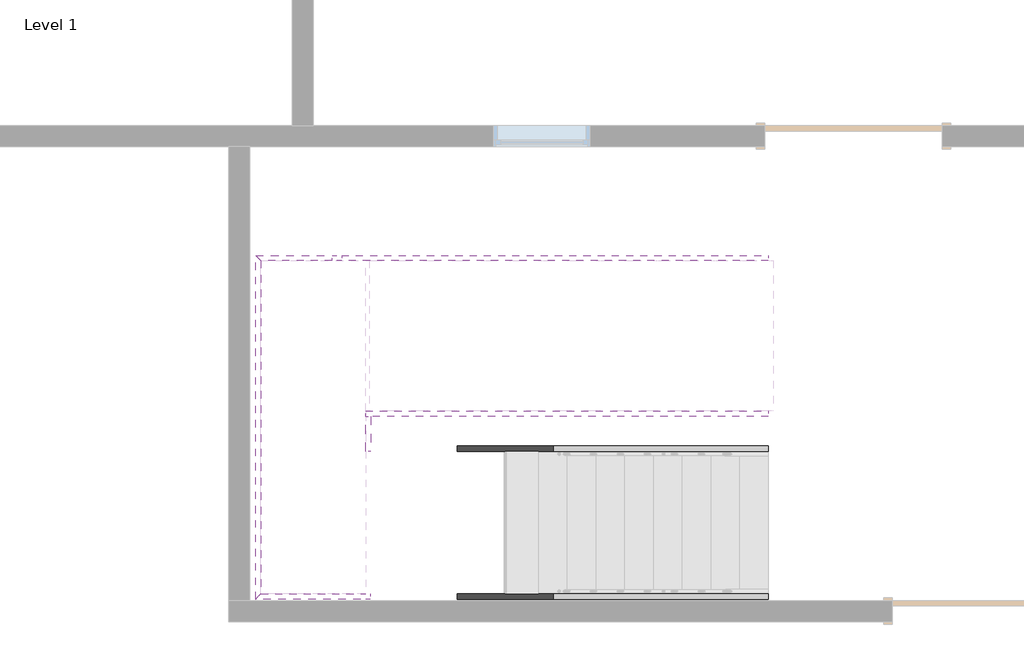
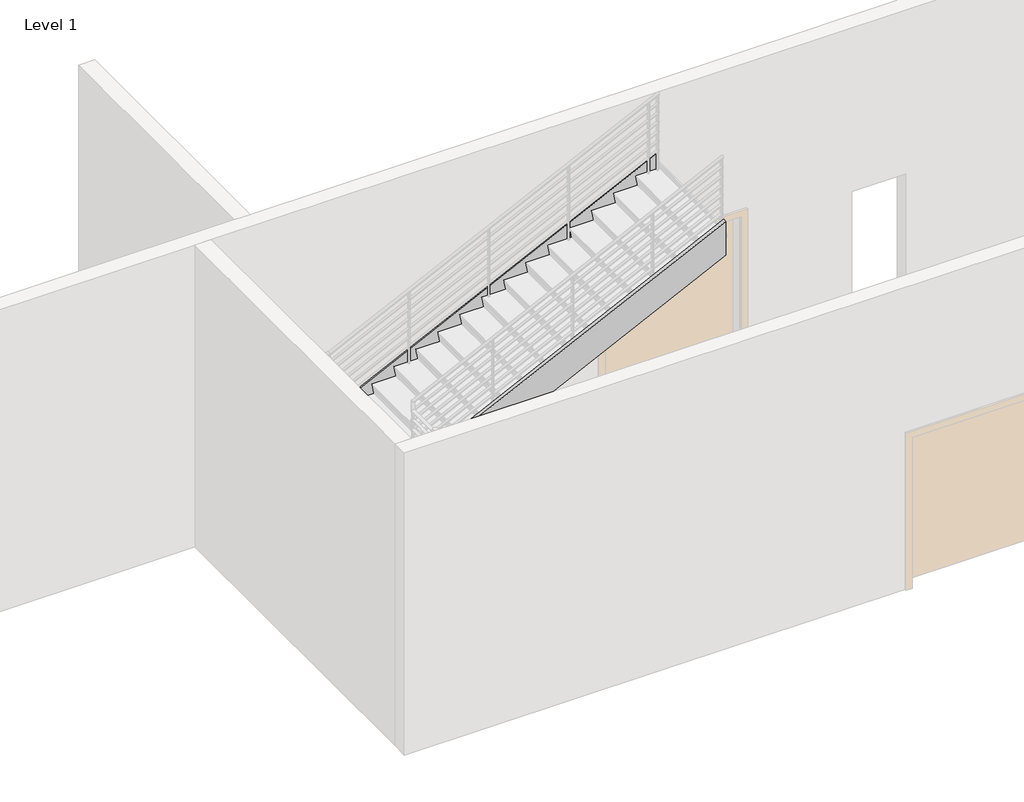
# One storey, part 4 of 4: 8 members.
"""IFC4 building model written with IfcOpenShell, lengths in millimetres."""

from ifc_helpers import new_model, si_unit, frame, origin, place, context, project, spatial, polyline, outline, extrude, faceted_brep, element, save

model = new_model("IFC4")

# Units and contexts
model_context = context("Model", 3, world=origin())
ifc_project = project(units=[si_unit("LENGTHUNIT", "METRE", prefix="MILLI")], contexts=[model_context])

# Site, building, storey
site = spatial("IfcSite", under=ifc_project)
building = spatial("IfcBuilding", under=site)
storey = spatial("IfcBuildingStorey", under=building, Name="Level 1", Elevation=0.0)

# Members
placement = place(None, origin())
element("IfcMember", 1, ObjectType="Stringer - 50mm Width", at=placement, inside=storey, context=model_context, shape_type="SweptSolid", body=[
    extrude(outline(polyline([(0.0, 3615.6033064), (202.7795961, 3615.6033064), (2047.393727, -188.9133386), (1647.393727, -280.7693796), (0.0, 3116.9801822), (0.0, 3615.6033064)])), frame((0.0, -1199.071626, 0.0), z_axis=(0.0, 1.0, 0.0), x_axis=(0.0, 0.0, 1.0)), (0.0, 0.0, 1.0), 50.0),
])
element("IfcMember", 2, ObjectType="Stringer - 50mm Width", at=placement, inside=storey, context=model_context, shape_type="SweptSolid", body=[
    extrude(outline(polyline([(0.0, 3615.6033064), (202.7795961, 3615.6033064), (2045.2038385, -184.3966936), (1600.6675762, -184.3966936), (0.0, 3116.9801822), (0.0, 3615.6033064)])), frame((0.0, 215.3469597, 0.0), z_axis=(0.0, 1.0, 0.0), x_axis=(0.0, 0.0, 1.0)), (0.0, 0.0, 1.0), 50.0),
])
element("IfcMember", 3, ObjectType="Stringer - 50mm Width", at=placement, inside=storey, context=model_context, shape_type="SweptSolid", body=[
    extrude(outline(polyline([(2047.393727, -554.8800486), (1647.393727, -463.0240075), (3624.9100004, 3615.6033064), (4069.4462627, 3615.6033064), (2047.393727, -554.8800486)])), frame((0.0, 2038.4290713, 0.0), z_axis=(0.0, 1.0, 0.0), x_axis=(0.0, 0.0, 1.0)), (0.0, 0.0, 1.0), 50.0),
])
element("IfcMember", 4, ObjectType="Stringer - 50mm Width", at=placement, inside=storey, context=model_context, shape_type="SweptSolid", body=[
    extrude(outline(polyline([(2202.7795961, -234.3966936), (1758.2433337, -234.3966936), (3624.9100004, 3615.6033064), (4069.4462627, 3615.6033064), (2202.7795961, -234.3966936)])), frame((0.0, 551.2300402, 0.0), z_axis=(0.0, 1.0, 0.0), x_axis=(0.0, 0.0, 1.0)), (0.0, 0.0, 1.0), 50.0),
])
element("IfcMember", 5, ObjectType="Stringer - 50mm Width", at=placement, inside=storey, context=model_context, shape_type="Brep", body=[
    faceted_brep([(-554.8800486, 2038.4290713, 2047.393727), (-554.8800486, 2088.4290713, 2047.393727), (-1284.4224748, 2088.4290713, 2047.393727), (-1234.4224748, 2038.4290713, 2047.393727), (-463.0240075, 2038.4290713, 1647.393727), (-1234.4224748, 2038.4290713, 1647.393727), (-463.0240075, 2088.4290713, 1647.393727), (-1284.4224748, 2088.4290713, 1647.393727)], [[[0, 1, 2, 3]], [[4, 0, 3, 5]], [[6, 4, 5, 7]], [[1, 6, 7, 2]], [[1, 0, 4, 6]], [[2, 7, 5, 3]]]),
])
element("IfcMember", 6, ObjectType="Stringer - 50mm Width", at=placement, inside=storey, context=model_context, shape_type="SweptSolid", body=[
    extrude(outline(polyline([(-1284.4224748, 2088.4290713), (-1234.4224748, 2038.4290713), (-1234.4224748, -1149.071626), (-1284.4224748, -1199.071626), (-1284.4224748, 2088.4290713)])), frame((0.0, 0.0, 1647.393727), z_axis=(0.0, 0.0, 1.0), x_axis=(1.0, 0.0, 0.0)), (0.0, 0.0, 1.0), 400.0),
])
element("IfcMember", 7, ObjectType="Stringer - 50mm Width", at=placement, inside=storey, context=model_context, shape_type="Brep", body=[
    faceted_brep([(-1234.4224748, -1149.071626, 2047.393727), (-1284.4224748, -1199.071626, 2047.393727), (-188.9133386, -1199.071626, 2047.393727), (-188.9133386, -1149.071626, 2047.393727), (-1234.4224748, -1149.071626, 1647.393727), (-280.7693796, -1149.071626, 1647.393727), (-1284.4224748, -1199.071626, 1647.393727), (-280.7693796, -1199.071626, 1647.393727)], [[[0, 1, 2, 3]], [[4, 0, 3, 5]], [[6, 4, 5, 7]], [[1, 6, 7, 2]], [[1, 0, 4, 6]], [[2, 7, 5, 3]]]),
])
element("IfcMember", 8, ObjectType="Stringer - 50mm Width", at=placement, inside=storey, context=model_context, shape_type="SweptSolid", body=[
    extrude(outline(polyline([(-184.3966936, 215.3469597), (-234.3966936, 215.3469597), (-234.3966936, 551.2300402), (-184.3966936, 551.2300402), (-184.3966936, 215.3469597)])), frame((0.0, 0.0, 1647.393727), z_axis=(0.0, 0.0, 1.0), x_axis=(1.0, 0.0, 0.0)), (0.0, 0.0, 1.0), 400.0),
])

save(model, "model.ifc")

# Revit data of these elements
# Elements 1, 2, 3, 4, 5, 6, 7, 8 (IfcMember, "Stringer - 50mm Width")
#   Phase Created = New Construction
